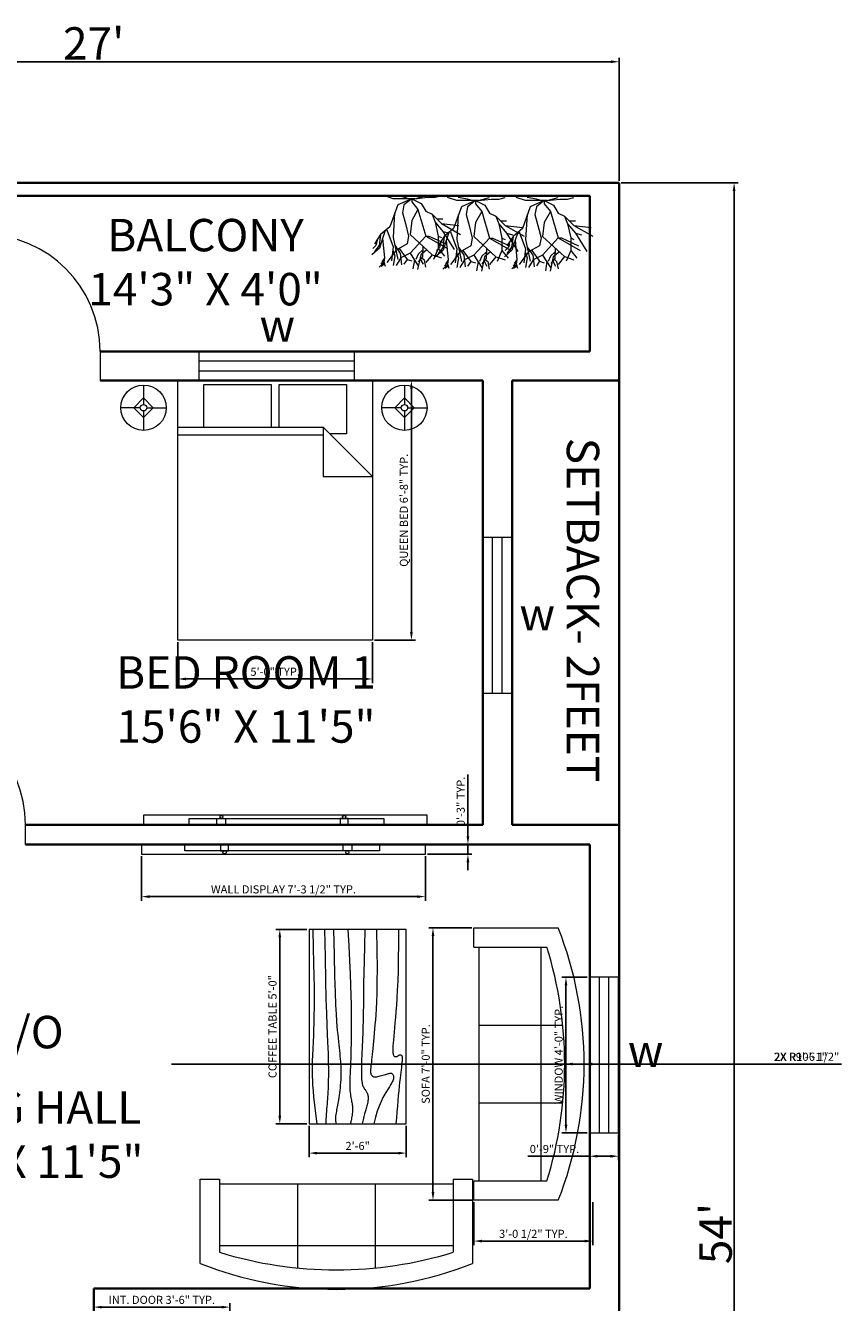
# Model space of a CAD drawing. Units: inches. Extents: x 2729 to 3178, y 5006 to 5809.
# Tile 4 of 4: x 2889 to 3141, y 5415 to 5809. Entities that reach past the tile are written whole.
import ezdxf

# ---------------------------------------------------------------- set-up
doc = ezdxf.new("R2010")
doc.units = ezdxf.units.IN
doc.layers.get('Defpoints').update_dxf_attribs({"color": 72})
for name, color, linetype, lineweight in [('A-ANNO-DIMS', 2, 'Continuous', 18), ('A-ANNO-TEXT', 7, 'Continuous', 18), ('A-AREA-IDEN', 7, 'Continuous', 25), ('A-DOOR', 4, 'Continuous', 18), ('A-EQPM', 8, 'Continuous', 18), ('A-FURN', 8, 'Continuous', 18), ('A-GLAZ', 4, 'Continuous', 18), ('A-WALL', 7, 'Continuous', 35), ('L-PLNT', 72, 'Continuous', 13)]:
    doc.layers.add(name, color=color, linetype=linetype, lineweight=lineweight)
doc.styles.get("Standard").update_dxf_attribs({"font": 'arial.ttf'})
doc.dimstyles.new('ISO-25', dxfattribs={"dimtxt": 2.5, "dimasz": 2.5, "dimexe": 1.25, "dimexo": 0.625, "dimtad": 1, "dimdec": 0, "dimlunit": 3, "dimtxsty": 'Standard', "dimcen": 2.5, "dimadec": 0, "dimazin": 0, "dimtfac": 1, "dimtdec": 0, "dimtmove": 0, "dimatfit": 3, "dimfxl": 1, "dimarcsym": 0})

# ---------------------------------------------------------------- blocks, each defined once
blk = doc.blocks.new('*D1')
at = {"layer": 'A-ANNO-DIMS', "color": 0, "lineweight": -2, "transparency": 16777216}
for p, q in [((2748.18, 5761.26), (2748.18, 5799.21)), ((2750.68, 5797.96), (3069.68, 5797.96)), ((3072.18, 5761.26), (3072.18, 5799.21))]:
    blk.add_line(p, q, dxfattribs=at)
at = {"layer": 'A-ANNO-DIMS', "color": 0, "transparency": 16777216}
for points in [[(2750.68, 5798.38), (2750.68, 5797.54), (2748.18, 5797.96)], [(3069.68, 5798.38), (3069.68, 5797.54), (3072.18, 5797.96)]]:
    blk.add_solid(points, dxfattribs=at)
at = {"layer": 'Defpoints', "color": 0, "transparency": 16777216}
for p in [(3072.18, 5797.96), (2748.18, 5760.64), (3072.18, 5760.64)]:
    blk.add_point(p, dxfattribs=at)
at = {"layer": 'A-ANNO-DIMS', "color": 0, "transparency": 16777216, "insert": (2910.18, 5803.61), "char_height": 2.5, "attachment_point": 5}
blk.add_mtext("{\\H4x;27'}", dxfattribs=at)
blk = doc.blocks.new('*D2')
at = {"layer": 'A-ANNO-DIMS', "color": 0, "lineweight": -2, "transparency": 16777216}
for p, q in [((3072.8, 5760.64), (3108.86, 5760.64)), ((3107.61, 5758.14), (3107.61, 5115.14)), ((3072.8, 5112.64), (3108.86, 5112.64))]:
    blk.add_line(p, q, dxfattribs=at)
at = {"layer": 'A-ANNO-DIMS', "color": 0, "transparency": 16777216}
for points in [[(3107.19, 5758.14), (3108.02, 5758.14), (3107.61, 5760.64)], [(3107.19, 5115.14), (3108.02, 5115.14), (3107.61, 5112.64)]]:
    blk.add_solid(points, dxfattribs=at)
at = {"layer": 'Defpoints', "color": 0, "transparency": 16777216}
for p in [(3072.18, 5760.64), (3072.18, 5112.64), (3107.61, 5112.64)]:
    blk.add_point(p, dxfattribs=at)
at = {"layer": 'A-ANNO-DIMS', "color": 0, "transparency": 16777216, "insert": (3101.9, 5436.64), "char_height": 2.5, "attachment_point": 5, "rotation": 90}
blk.add_mtext("{\\H4x;54'}", dxfattribs=at)
blk = doc.blocks.new('Sofa - Roundback 7 ft.')
for p, q in [((-12.00002, -32.4421), (-12.00003, -6.5971)), ((11.99997, -32.4421), (11.99998, -6.5971)), ((-36.000027, -34), (-36.000027, -11.4696)), ((35.99998, -34), (35.99998, -11.4696)), ((-35.999844, -13.3819), (35.9998, -13.3819)), ((-36.000027, -32.4421), (35.99998, -32.4421))]:
    blk.add_line(p, q)
for points in [[(-36.000027, -34), (-42.000027, -34), (-42.000027, -8)], [(41.99998, -8), (41.99998, -34), (35.99998, -34)]]:
    blk.add_lwpolyline(points)
for centre, radius, start, end in [((0, -114.25), 114.25, 68.43141, 111.5686), ((-0.00001, -127.1968), 121.1968, 72.72033, 107.2797)]:
    blk.add_arc(centre, radius, start, end)
blk = doc.blocks.new('Table - Rectangular Woodgrain 60 x 30 in.')
for p, q in [((0, 0), (0, -30)), ((60, 0), (0, 0)), ((60, -30), (60, 0)), ((0, -30), (60, -30))]:
    blk.add_line(p, q)
for points in [[(0, -2.4), (4.8155, -2.418), (9.0302, -2.4688), (12.709, -2.5477), (15.9167, -2.65), (18.7181, -2.7711), (21.1781, -2.9063), (23.3616, -3.0508), (25.3333, -3.2), (27.1477, -3.3495), (28.8172, -3.4958), (30.3437, -3.636), (31.7291, -3.7667), (32.9756, -3.8849), (34.0849, -3.9875), (35.059, -4.0714), (35.9, -4.1334), (36.6114, -4.1711), (37.2041, -4.1854), (37.6906, -4.1779), (38.0833, -4.15), (38.3948, -4.1034), (38.6375, -4.0396), (38.8239, -3.9602), (38.9666, -3.8667), (39.0764, -3.7608), (39.1573, -3.6448), (39.2116, -3.521), (39.2416, -3.3917), (39.2498, -3.2593), (39.2385, -3.1261), (39.21, -2.9944), (39.1666, -2.8667), (39.111, -2.7447), (39.0468, -2.6281), (38.978, -2.5163), (38.9083, -2.4083), (38.8418, -2.3035), (38.7823, -2.201), (38.7337, -2.1001), (38.7, -2), (38.6844, -1.9003), (38.6875, -1.8021), (38.7094, -1.707), (38.75, -1.6167), (38.8094, -1.5326), (38.8875, -1.4563), (38.9844, -1.3893), (39.1, -1.3333), (39.2351, -1.2896), (39.3937, -1.2583), (39.5804, -1.2396), (39.8, -1.2333), (40.057, -1.2396), (40.3562, -1.2583), (40.7023, -1.2896), (41.1, -1.3333), (41.5547, -1.3895), (42.0755, -1.4573), (42.6721, -1.5361), (43.3542, -1.625), (44.1316, -1.7233), (45.014, -1.8302), (46.0114, -1.9449), (47.1333, -2.0667), (48.3862, -2.1947), (49.7625, -2.3281), (51.2513, -2.4663), (52.8416, -2.6083), (54.5226, -2.7535), (56.2833, -2.9011), (58.1127, -3.0501), (60, -3.2)], [(0, -9.2), (6.5759, -9.0858), (11.9385, -9.0365), (16.2527, -9.0418), (19.6833, -9.0917), (22.3952, -9.1759), (24.5531, -9.2844), (26.322, -9.4069), (27.8666, -9.5333), (29.3241, -9.6553), (30.7203, -9.7719), (32.0532, -9.8837), (33.3208, -9.9917), (34.5213, -10.0965), (35.6526, -10.199), (36.7128, -10.2999), (37.7, -10.4), (38.6129, -10.4996), (39.4531, -10.5969), (40.223, -10.6895), (40.925, -10.775), (41.5613, -10.8512), (42.1344, -10.9156), (42.6465, -10.966), (43.1, -11), (43.4976, -11.0158), (43.8437, -11.0136), (44.143, -10.9942), (44.4, -10.9583), (44.6195, -10.9069), (44.8062, -10.8406), (44.9648, -10.7603), (45.1, -10.6667), (45.2155, -10.5598), (45.3114, -10.4365), (45.3871, -10.2929), (45.4416, -10.125), (45.4743, -9.929), (45.4844, -9.7011), (45.4709, -9.4371), (45.4333, -9.1333), (45.3716, -8.7883), (45.2896, -8.4104), (45.1919, -8.0107), (45.0833, -7.6), (44.9685, -7.1893), (44.8521, -6.7896), (44.7388, -6.4117), (44.6333, -6.0667), (44.54, -5.7628), (44.4614, -5.4979), (44.4001, -5.2675), (44.3583, -5.0667), (44.3384, -4.8909), (44.3427, -4.7354), (44.3736, -4.5956), (44.4333, -4.4667), (44.5236, -4.3453), (44.6427, -4.2333), (44.7884, -4.1339), (44.9583, -4.05), (45.1501, -3.9849), (45.3614, -3.9417), (45.59, -3.9234), (45.8333, -3.9333), (46.0915, -3.9749), (46.3734, -4.0531), (46.6906, -4.1736), (47.0542, -4.3417), (47.4756, -4.5629), (47.9661, -4.8427), (48.5372, -5.1866), (49.2, -5.6), (49.9676, -6.0844), (50.8594, -6.625), (51.8965, -7.2031), (53.1, -7.8), (54.491, -8.3969), (56.0906, -8.975), (57.9199, -9.5156), (60, -10)], [(0, -12.8), (5.1847, -12.9322), (9.6213, -13.0323), (13.3963, -13.1059), (16.5958, -13.1583), (19.3063, -13.1952), (21.614, -13.2219), (23.6054, -13.2439), (25.3666, -13.2667), (26.9728, -13.2947), (28.4531, -13.3281), (29.8256, -13.3663), (31.1083, -13.4083), (32.3191, -13.4535), (33.476, -13.501), (34.597, -13.5501), (35.7, -13.6), (36.7984, -13.6497), (37.8875, -13.6979), (38.9578, -13.743), (40, -13.7833), (41.0047, -13.8174), (41.9625, -13.8438), (42.864, -13.8607), (43.7, -13.8667), (44.4631, -13.8604), (45.1552, -13.8417), (45.7801, -13.8104), (46.3416, -13.7667), (46.8439, -13.7104), (47.2906, -13.6417), (47.6858, -13.5604), (48.0333, -13.4667), (48.3375, -13.3608), (48.6042, -13.2448), (48.8396, -13.121), (49.05, -12.9917), (49.2417, -12.8593), (49.4208, -12.7261), (49.5937, -12.5944), (49.7667, -12.4667), (49.9452, -12.3451), (50.1323, -12.2313), (50.3303, -12.1268), (50.5416, -12.0333), (50.7686, -11.9524), (51.0135, -11.8854), (51.2788, -11.8341), (51.5666, -11.8), (51.8785, -11.7843), (52.2116, -11.7865), (52.562, -11.8059), (52.926, -11.8417), (53.2998, -11.8931), (53.6795, -11.9594), (54.0614, -12.0397), (54.4416, -12.1333), (54.8223, -12.2401), (55.2293, -12.3625), (55.6942, -12.5037), (56.2489, -12.6667), (56.9251, -12.8547), (57.7545, -13.0708), (58.7689, -13.3182), (60, -13.6)], [(0, -18), (5.124, -17.7273), (9.6609, -17.5057), (13.6705, -17.3303), (17.2125, -17.1958), (20.3467, -17.0973), (23.1328, -17.0297), (25.6307, -16.9878), (27.9, -16.9667), (29.9928, -16.9617), (31.9302, -16.9703), (33.7254, -16.9907), (35.3917, -17.0208), (36.9423, -17.0588), (38.3906, -17.1026), (39.7499, -17.1503), (41.0333, -17.2), (42.2519, -17.2496), (43.4073, -17.2969), (44.4986, -17.3395), (45.525, -17.375), (46.4858, -17.4012), (47.3802, -17.4156), (48.2074, -17.416), (48.9667, -17.4), (49.6583, -17.3662), (50.2872, -17.3167), (50.8595, -17.2547), (51.3812, -17.1833), (51.8584, -17.1057), (52.2971, -17.025), (52.7034, -16.9443), (53.0833, -16.8667), (53.443, -16.7951), (53.789, -16.7313), (54.128, -16.6768), (54.4666, -16.6334), (54.8115, -16.6024), (55.1693, -16.5854), (55.5465, -16.5841), (55.95, -16.6), (56.3828, -16.6337), (56.8346, -16.6823), (57.2915, -16.7418), (57.7396, -16.8084), (58.165, -16.878), (58.5539, -16.9469), (58.8924, -17.0111), (59.1666, -17.0667), (59.3679, -17.1107), (59.5078, -17.1438), (59.6032, -17.1675), (59.6708, -17.1833), (59.7275, -17.193), (59.7901, -17.1979), (59.8753, -17.1998), (60, -17.2)], [(0, -22.4), (8.0098, -22.2501), (14.4094, -22.1011), (19.4168, -21.9535), (23.25, -21.8083), (26.1269, -21.6663), (28.2656, -21.5281), (29.884, -21.3947), (31.2, -21.2667), (32.3967, -21.1448), (33.5172, -21.0292), (34.5697, -20.9198), (35.5625, -20.8167), (36.5037, -20.7198), (37.4015, -20.6292), (38.2642, -20.5448), (39.1, -20.4667), (39.9164, -20.3951), (40.7187, -20.3313), (41.5117, -20.2768), (42.3, -20.2333), (43.0883, -20.2024), (43.8812, -20.1854), (44.6836, -20.1841), (45.5, -20.2), (46.3328, -20.234), (47.1747, -20.2844), (48.0163, -20.3488), (48.8479, -20.425), (49.66, -20.5106), (50.4429, -20.6031), (51.1872, -20.7004), (51.8833, -20.8), (52.5246, -20.8999), (53.1166, -20.9995), (53.6681, -21.0983), (54.1875, -21.1958), (54.6834, -21.2919), (55.1646, -21.3859), (55.6394, -21.4777), (56.1167, -21.5667), (56.6028, -21.6515), (57.0961, -21.7266), (57.5929, -21.7852), (58.0896, -21.8208), (58.5823, -21.8268), (59.0674, -21.7964), (59.5412, -21.723), (60, -21.6)], [(0, -25.2), (8.6355, -25.0504), (15.7026, -24.9031), (21.4049, -24.7606), (25.9458, -24.625), (29.529, -24.4988), (32.3578, -24.3844), (34.6359, -24.284), (36.5667, -24.2), (38.3213, -24.1341), (39.9417, -24.0854), (41.437, -24.0523), (42.8167, -24.0333), (44.0901, -24.0268), (45.2667, -24.0313), (46.3557, -24.0451), (47.3667, -24.0667), (48.309, -24.0947), (49.1928, -24.1287), (50.0284, -24.168), (50.826, -24.2125), (51.5959, -24.2617), (52.3483, -24.3151), (53.0935, -24.3725), (53.8417, -24.4334), (54.6009, -24.497), (55.3699, -24.561), (56.1454, -24.6226), (56.9239, -24.6792), (57.7021, -24.7279), (58.4764, -24.7662), (59.2435, -24.7911), (60, -24.8)], [(0, -28.8), (5.6867, -28.6681), (10.45, -28.5698), (14.407, -28.5012), (17.675, -28.4584), (20.3711, -28.4374), (22.6125, -28.4344), (24.5164, -28.4455), (26.2, -28.4667), (27.762, -28.4947), (29.2276, -28.5281), (30.6033, -28.5663), (31.8958, -28.6084), (33.1118, -28.6535), (34.2578, -28.7011), (35.3405, -28.7501), (36.3666, -28.8), (37.3443, -28.8497), (38.288, -28.8974), (39.2137, -28.9412), (40.1375, -28.9792), (41.0753, -29.0093), (42.0432, -29.0297), (43.0572, -29.0384), (44.1333, -29.0333), (45.2936, -29.0114), (46.5843, -28.9641), (48.0579, -28.8816), (49.7666, -28.7542), (51.7629, -28.5721), (54.0989, -28.3255), (56.8272, -28.0048), (60, -27.6)]]:
    blk.add_lwpolyline(points)
blk = doc.blocks.new('Bed - Queen')
for p, q in [((0, -80.00003), (0, 0)), ((0, 0), (59.99999, 0)), ((59.99999, 0), (59.99999, -80.00003)), ((7.99999, -1.2), (28.79998, -1.2)), ((7.99999, -14.4), (7.99999, -1.2)), ((28.79998, -1.2), (28.79998, -14.4)), ((31.19999, -1.2), (51.99999, -1.2)), ((31.19999, -14.4), (31.19999, -1.2)), ((51.99999, -1.2), (51.99999, -16.4)), ((0, -14.4), (44.8, -14.4)), ((59.99999, -29.6), (44.8, -14.4)), ((44.8, -14.4), (44.8, -29.6)), ((44.8, -16.8), (0, -16.8)), ((51.99999, -16.4), (46.79936, -16.4)), ((44.8, -29.6), (59.99999, -29.6)), ((59.99999, -80.00003), (0, -80.00003))]:
    blk.add_line(p, q)
blk = doc.blocks.new('Lamp - Table')
for p, q in [((0, 7), (0, 1)), ((-1, 0), (-7, 0)), ((0, 3), (-3, 0)), ((-3, 0), (0, -3)), ((3, 0), (0, 3)), ((0, -3), (3, 0)), ((1, 0), (7, 0)), ((0, -1), (0, -7))]:
    blk.add_line(p, q)
for radius in [7, 1]:
    blk.add_circle((0, 0), radius)
blk = doc.blocks.new('*U13')
for p, q in [((-377.952, 463.296), (-329.184, 524.256)), ((-316.7634, 502.285), (-327.6092, 559.9176)), ((-296.5958, 484.4034), (-316.7634, 502.285)), ((-286.512, 498.3226), (-307.4416, 538.0736)), ((-302.7934, 478.4344), (-270.256, 518.1854)), ((-290.3982, 464.5406), (-265.6078, 577.8246)), ((-268.7066, 458.5716), (-250.0884, 500.3038)), ((-207.264, 451.104), (-268.224, 548.64)), ((-240.792, 502.285), (-228.3968, 573.8368)), ((-182.88, 499.872), (-219.456, 512.064)), ((-182.88, 499.872), (-158.496, 536.448)), ((-129.1844, 450.6214), (-140.0302, 542.036)), ((-134.112, 487.68), (-97.536, 548.64)), ((-97.536, 426.72), (-24.384, 524.256)), ((-85.7758, 472.4908), (-73.3552, 548.005)), ((-73.152, 402.336), (-60.96, 512.064)), ((-12.9032, 555.9552), (-2.0574, 522.1732)), ((-5.1562, 486.3846), (2.5908, 542.036)), ((-3.6068, 492.3536), (14.986, 518.1854)), ((-0.508, 508.254), (22.7584, 536.067)), ((1.0414, 526.1356), (35.1536, 559.9176)), ((2.5908, 542.036), (21.209, 555.9552)), ((-463.296, 280.416), (-552.577, 423.037)), ((-329.184, 316.992), (-499.872, 414.528)), ((-426.72, 414.528), (-475.488, 475.488)), ((-377.952, 463.296), (-451.104, 487.68)), ((-426.72, 414.528), (-390.144, 499.872)), ((-426.72, 316.992), (-426.72, 414.528)), ((-207.264, 304.8), (-377.952, 463.296)), ((-338.455, 424.7896), (-290.3982, 464.5406)), ((-329.184, 316.992), (-207.264, 451.104)), ((-305.8922, 396.9512), (-302.7934, 478.4344)), ((-304.3428, 426.7708), (-268.7066, 458.5716)), ((-207.264, 451.104), (-134.112, 487.68)), ((-121.92, 414.528), (-182.88, 499.872)), ((-182.88, 377.952), (-97.536, 426.72)), ((-85.7758, 389.001), (-129.1844, 452.6026)), ((-73.152, 329.184), (-109.728, 499.872)), ((-70.2564, 426.7708), (-85.7758, 472.4908)), ((-24.384, 268.224), (-73.152, 402.336)), ((8.7884, 335.3562), (-5.1562, 486.3846)), ((8.7884, 335.3562), (33.6042, 412.8516)), ((33.6042, 412.8516), (92.5068, 464.5406)), ((36.576, 390.144), (73.152, 438.912)), ((60.96, 390.144), (85.344, 414.528)), ((-451.104, 219.456), (-601.0402, 303.8094)), ((-353.568, 316.992), (-487.68, 377.952)), ((-426.72, 316.992), (-451.104, 329.184)), ((-402.336, 207.264), (-426.72, 316.992)), ((-329.184, 316.992), (-353.568, 316.992)), ((-268.224, 109.728), (-329.184, 316.992)), ((-219.456, 195.072), (-207.264, 304.8)), ((-195.072, 316.992), (-182.88, 377.952)), ((-170.688, 219.456), (-195.072, 316.992)), ((-85.344, 134.112), (-73.152, 329.184)), ((-48.768, 243.84), (24.384, 304.8)), ((-12.192, 274.32), (8.7884, 335.3562)), ((24.384, 304.8), (36.576, 390.144)), ((24.384, 304.8), (73.152, 377.952)), ((48.768, 341.376), (60.96, 390.144)), ((-451.104, 219.456), (-587.4512, 234.2388)), ((-463.296, 280.416), (-512.064, 292.608)), ((-402.336, 207.264), (-463.296, 280.416)), ((-377.952, 146.304), (-451.104, 219.456)), ((-377.952, 146.304), (-402.336, 207.264)), ((-146.304, 134.112), (-170.688, 219.456)), ((-109.728, 73.152), (-48.768, 243.84)), ((-414.528, 182.88), (-463.296, 182.88)), ((-329.184, 121.92), (-377.952, 146.304)), ((-292.608, 60.96), (-329.184, 121.92)), ((-268.224, 109.728), (-219.456, 195.072)), ((-219.456, 48.768), (-268.224, 109.728)), ((-158.496, 73.152), (-146.304, 134.112)), ((-402.336, 12.192), (-451.104, 0)), ((-341.376, 12.192), (-402.336, 12.192)), ((-243.84, 24.384), (-341.376, 12.192)), ((-243.84, 24.384), (-329.184, 0)), ((-219.456, 24.384), (-292.608, 60.96)), ((-243.84, 24.384), (-195.072, 24.384)), ((-219.456, 24.384), (-109.728, 73.152)), ((-219.456, 24.384), (-158.496, 73.152)), ((-219.456, 24.384), (-219.456, 48.768)), ((-219.456, 24.384), (-73.152, 24.384)), ((-195.072, 24.384), (-158.496, 12.192)), ((-158.496, 12.192), (-85.344, 0)), ((-73.152, 24.384), (0, 0))]:
    blk.add_line(p, q)
blk = doc.blocks.new('WIN-48IN')
for p, q in [((48, 9), (0, 9)), ((0, 9), (0, 0)), ((48, 0), (48, 9)), ((48, 6), (0, 6)), ((0, 3), (48, 3)), ((0, 0), (48, 0))]:
    blk.add_line(p, q)
blk = doc.blocks.new('DISPLAY-WALL-60IN')
for p, q in [((0, 3), (0, 0)), ((13.37, 1), (13.37, 3)), ((13.37, 3), (73.37, 3)), ((73.37, 1), (13.37, 1)), ((24.34, 3), (24.34, 1)), ((24.34, 1), (26.79, 1)), ((26.79, 1), (26.79, 3)), ((62.14, 1), (62.14, 3)), ((64.8, 1), (62.14, 1)), ((64.8, 3), (64.8, 1)), ((73.37, 3), (73.37, 1)), ((87.48, 0), (87.48, 3)), ((0, 0), (87.48, 0))]:
    blk.add_line(p, q)
for centre, radius in [((25.58, 0.52), 0.492), ((63.4, 0.52), 0.473)]:
    blk.add_circle(centre, radius)
blk = doc.blocks.new('DOOR-36IN-JAMB6')
for p, q in [((0, 6), (0, 42)), ((1, 6), (1, 42)), ((0, 6), (0, 0)), ((1, 6), (1, 0)), ((36, 0), (36, 6))]:
    blk.add_line(p, q)
blk.add_arc((0, 6), 36, 0, 90)
blk = doc.blocks.new('*D27')
at = {"layer": 'A-ANNO-DIMS', "color": 0, "lineweight": -2, "transparency": 16777216}
for p, q in [((3062.36, 5515.67), (3054.53, 5515.67)), ((3055.78, 5470.17), (3055.78, 5513.17)), ((3062.36, 5467.67), (3054.53, 5467.67))]:
    blk.add_line(p, q, dxfattribs=at)
at = {"layer": 'A-ANNO-DIMS', "color": 0, "transparency": 16777216}
for points in [[(3055.37, 5513.17), (3056.2, 5513.17), (3055.78, 5515.67)], [(3055.37, 5470.17), (3056.2, 5470.17), (3055.78, 5467.67)]]:
    blk.add_solid(points, dxfattribs=at)
at = {"layer": 'Defpoints', "color": 0, "transparency": 16777216}
for p in [(3055.78, 5515.67), (3062.98, 5515.67), (3062.98, 5467.67)]:
    blk.add_point(p, dxfattribs=at)
at = {"layer": 'A-ANNO-DIMS', "color": 0, "transparency": 16777216, "insert": (3053.86, 5491.67), "char_height": 2.5, "attachment_point": 5, "rotation": 90}
blk.add_mtext('WINDOW 4\'-0" TYP.', dxfattribs=at)
blk = doc.blocks.new('*D28')
at = {"layer": 'A-ANNO-DIMS', "color": 0, "lineweight": -2, "transparency": 16777216}
for p, q in [((3062.98, 5467.04), (3062.98, 5459.22)), ((3071.98, 5467.04), (3071.98, 5459.22)), ((3062.98, 5460.47), (3043.99, 5460.47)), ((3069.48, 5460.47), (3065.48, 5460.47))]:
    blk.add_line(p, q, dxfattribs=at)
at = {"layer": 'A-ANNO-DIMS', "color": 0, "transparency": 16777216}
for points in [[(3065.48, 5460.89), (3065.48, 5460.05), (3062.98, 5460.47)], [(3069.48, 5460.89), (3069.48, 5460.05), (3071.98, 5460.47)]]:
    blk.add_solid(points, dxfattribs=at)
at = {"layer": 'Defpoints', "color": 0, "transparency": 16777216}
for p in [(3062.98, 5467.67), (3071.98, 5467.67), (3062.98, 5460.47)]:
    blk.add_point(p, dxfattribs=at)
at = {"layer": 'A-ANNO-DIMS', "color": 0, "transparency": 16777216, "insert": (3052.24, 5462.37), "char_height": 2.5, "attachment_point": 5}
blk.add_mtext('0\'-9" TYP.', dxfattribs=at)
blk = doc.blocks.new('*D31')
at = {"layer": 'A-ANNO-DIMS', "color": 0, "lineweight": -2, "transparency": 16777216}
for p, q in [((2996.75, 5699.64), (3009.38, 5699.64)), ((3008.13, 5622.14), (3008.13, 5697.14)), ((2996.75, 5619.64), (3009.38, 5619.64))]:
    blk.add_line(p, q, dxfattribs=at)
at = {"layer": 'A-ANNO-DIMS', "color": 0, "transparency": 16777216}
for points in [[(3007.71, 5697.14), (3008.55, 5697.14), (3008.13, 5699.64)], [(3007.71, 5622.14), (3008.55, 5622.14), (3008.13, 5619.64)]]:
    blk.add_solid(points, dxfattribs=at)
at = {"layer": 'Defpoints', "color": 0, "transparency": 16777216}
for p in [(2996.13, 5699.64), (3008.13, 5699.64), (2996.13, 5619.64)]:
    blk.add_point(p, dxfattribs=at)
at = {"layer": 'A-ANNO-DIMS', "color": 0, "transparency": 16777216, "insert": (3006.13, 5659.64), "char_height": 2.5, "attachment_point": 5, "rotation": 90}
blk.add_mtext('QUEEN BED 6\'-8" TYP.', dxfattribs=at)
blk = doc.blocks.new('*D32')
at = {"layer": 'A-ANNO-DIMS', "color": 0, "lineweight": -2, "transparency": 16777216}
for p, q in [((2936.13, 5619.01), (2936.13, 5606.39)), ((2996.13, 5619.01), (2996.13, 5606.39)), ((2938.63, 5607.64), (2993.63, 5607.64))]:
    blk.add_line(p, q, dxfattribs=at)
at = {"layer": 'A-ANNO-DIMS', "color": 0, "transparency": 16777216}
for points in [[(2938.63, 5608.05), (2938.63, 5607.22), (2936.13, 5607.64)], [(2993.63, 5608.05), (2993.63, 5607.22), (2996.13, 5607.64)]]:
    blk.add_solid(points, dxfattribs=at)
at = {"layer": 'Defpoints', "color": 0, "transparency": 16777216}
for p in [(2936.13, 5619.64), (2996.13, 5619.64), (2996.13, 5607.64)]:
    blk.add_point(p, dxfattribs=at)
at = {"layer": 'A-ANNO-DIMS', "color": 0, "transparency": 16777216, "insert": (2966.13, 5609.54), "char_height": 2.5, "attachment_point": 5}
blk.add_mtext('5\'-0" TYP.', dxfattribs=at)
blk = doc.blocks.new('*D35')
at = {"layer": 'A-ANNO-DIMS', "color": 0, "lineweight": -2, "transparency": 16777216}
for p, q in [((2910.18, 5408.26), (2910.18, 5415.19)), ((2952.18, 5408.26), (2952.18, 5415.19)), ((2912.68, 5413.94), (2949.68, 5413.94))]:
    blk.add_line(p, q, dxfattribs=at)
at = {"layer": 'A-ANNO-DIMS', "color": 0, "transparency": 16777216}
for points in [[(2912.68, 5414.35), (2912.68, 5413.52), (2910.18, 5413.94)], [(2949.68, 5414.35), (2949.68, 5413.52), (2952.18, 5413.94)]]:
    blk.add_solid(points, dxfattribs=at)
at = {"layer": 'Defpoints', "color": 0, "transparency": 16777216}
for p in [(2952.18, 5413.94), (2910.18, 5407.64), (2952.18, 5407.64)]:
    blk.add_point(p, dxfattribs=at)
at = {"layer": 'A-ANNO-DIMS', "color": 0, "transparency": 16777216, "insert": (2931.18, 5415.86), "char_height": 2.5, "attachment_point": 5}
blk.add_mtext('INT. DOOR 3\'-6" TYP.', dxfattribs=at)
blk = doc.blocks.new('*D37')
at = {"layer": 'A-ANNO-DIMS', "color": 0, "lineweight": -2, "transparency": 16777216}
for p, q in [((3026.76, 5530.9), (3013.53, 5530.9)), ((3014.78, 5528.4), (3014.78, 5449.4)), ((3026.76, 5446.9), (3013.53, 5446.9))]:
    blk.add_line(p, q, dxfattribs=at)
at = {"layer": 'A-ANNO-DIMS', "color": 0, "transparency": 16777216}
for points in [[(3014.37, 5528.4), (3015.2, 5528.4), (3014.78, 5530.9)], [(3014.37, 5449.4), (3015.2, 5449.4), (3014.78, 5446.9)]]:
    blk.add_solid(points, dxfattribs=at)
at = {"layer": 'Defpoints', "color": 0, "transparency": 16777216}
for p in [(3027.38, 5530.9), (3014.78, 5446.9), (3027.38, 5446.9)]:
    blk.add_point(p, dxfattribs=at)
at = {"layer": 'A-ANNO-DIMS', "color": 0, "transparency": 16777216, "insert": (3012.87, 5488.9), "char_height": 2.5, "attachment_point": 5, "rotation": 90}
blk.add_mtext('SOFA 7\'-0" TYP.', dxfattribs=at)
blk = doc.blocks.new('*D38')
at = {"layer": 'A-ANNO-DIMS', "color": 0, "lineweight": -2, "transparency": 16777216}
for p, q in [((3027.38, 5446.27), (3027.38, 5433.05)), ((3064.05, 5446.27), (3064.05, 5433.05)), ((3029.88, 5434.3), (3061.55, 5434.3))]:
    blk.add_line(p, q, dxfattribs=at)
at = {"layer": 'A-ANNO-DIMS', "color": 0, "transparency": 16777216}
for points in [[(3029.88, 5434.72), (3029.88, 5433.88), (3027.38, 5434.3)], [(3061.55, 5434.72), (3061.55, 5433.88), (3064.05, 5434.3)]]:
    blk.add_solid(points, dxfattribs=at)
at = {"layer": 'Defpoints', "color": 0, "transparency": 16777216}
for p in [(3027.38, 5446.9), (3064.05, 5446.9), (3064.05, 5434.3)]:
    blk.add_point(p, dxfattribs=at)
at = {"layer": 'A-ANNO-DIMS', "color": 0, "transparency": 16777216, "insert": (3045.72, 5436.22), "char_height": 2.5, "attachment_point": 5}
blk.add_mtext('3\'-0 1/2" TYP.', dxfattribs=at)
blk = doc.blocks.new('*D43')
at = {"layer": 'A-ANNO-DIMS', "color": 0, "lineweight": -2, "transparency": 16777216}
for p, q in [((2924.96, 5553.01), (2924.96, 5539.27)), ((3012.43, 5553.01), (3012.43, 5539.27)), ((2927.46, 5540.52), (3009.93, 5540.52))]:
    blk.add_line(p, q, dxfattribs=at)
at = {"layer": 'A-ANNO-DIMS', "color": 0, "transparency": 16777216}
for points in [[(2927.46, 5540.93), (2927.46, 5540.1), (2924.96, 5540.52)], [(3009.93, 5540.93), (3009.93, 5540.1), (3012.43, 5540.52)]]:
    blk.add_solid(points, dxfattribs=at)
at = {"layer": 'Defpoints', "color": 0, "transparency": 16777216}
for p in [(2924.96, 5553.64), (3012.43, 5553.64), (3012.43, 5540.52)]:
    blk.add_point(p, dxfattribs=at)
at = {"layer": 'A-ANNO-DIMS', "color": 0, "transparency": 16777216, "insert": (2968.69, 5542.43), "char_height": 2.5, "attachment_point": 5}
blk.add_mtext('WALL DISPLAY 7\'-3 1/2" TYP.', dxfattribs=at)
blk = doc.blocks.new('*D44')
at = {"layer": 'A-ANNO-DIMS', "color": 0, "lineweight": -2, "transparency": 16777216}
for p, q in [((3025.55, 5559.14), (3025.55, 5578.13)), ((3013.06, 5556.64), (3026.8, 5556.64)), ((3025.55, 5553.64), (3025.55, 5556.64)), ((3013.06, 5553.64), (3026.8, 5553.64)), ((3025.55, 5551.14), (3025.55, 5548.64))]:
    blk.add_line(p, q, dxfattribs=at)
at = {"layer": 'A-ANNO-DIMS', "color": 0, "transparency": 16777216}
for points in [[(3025.14, 5559.14), (3025.97, 5559.14), (3025.55, 5556.64)], [(3025.14, 5551.14), (3025.97, 5551.14), (3025.55, 5553.64)]]:
    blk.add_solid(points, dxfattribs=at)
at = {"layer": 'Defpoints', "color": 0, "transparency": 16777216}
for p in [(3012.43, 5556.64), (3025.55, 5556.64), (3012.43, 5553.64)]:
    blk.add_point(p, dxfattribs=at)
at = {"layer": 'A-ANNO-DIMS', "color": 0, "transparency": 16777216, "insert": (3023.65, 5569.88), "char_height": 2.5, "attachment_point": 5, "rotation": 90}
blk.add_mtext('0\'-3" TYP.', dxfattribs=at)
blk = doc.blocks.new('*D49')
at = {"layer": 'A-ANNO-DIMS', "color": 0, "lineweight": -2, "transparency": 16777216}
for p, q in [((2975.93, 5530.43), (2966.31, 5530.43)), ((2967.56, 5527.93), (2967.56, 5472.93)), ((2975.93, 5470.43), (2966.31, 5470.43))]:
    blk.add_line(p, q, dxfattribs=at)
at = {"layer": 'A-ANNO-DIMS', "color": 0, "transparency": 16777216}
for points in [[(2967.14, 5527.93), (2967.97, 5527.93), (2967.56, 5530.43)], [(2967.14, 5472.93), (2967.97, 5472.93), (2967.56, 5470.43)]]:
    blk.add_solid(points, dxfattribs=at)
at = {"layer": 'Defpoints', "color": 0, "transparency": 16777216}
for p in [(2976.56, 5530.43), (2967.56, 5470.43), (2976.56, 5470.43)]:
    blk.add_point(p, dxfattribs=at)
at = {"layer": 'A-ANNO-DIMS', "color": 0, "transparency": 16777216, "insert": (2965.64, 5500.43), "char_height": 2.5, "attachment_point": 5, "rotation": 90}
blk.add_mtext('COFFEE TABLE 5\'-0"', dxfattribs=at)
blk = doc.blocks.new('*D50')
at = {"layer": 'A-ANNO-DIMS', "color": 0, "lineweight": -2, "transparency": 16777216}
for p, q in [((2976.56, 5469.8), (2976.56, 5460.18)), ((3006.56, 5469.8), (3006.56, 5460.18)), ((2979.06, 5461.43), (3004.06, 5461.43))]:
    blk.add_line(p, q, dxfattribs=at)
at = {"layer": 'A-ANNO-DIMS', "color": 0, "transparency": 16777216}
for points in [[(2979.06, 5461.84), (2979.06, 5461.01), (2976.56, 5461.43)], [(3004.06, 5461.84), (3004.06, 5461.01), (3006.56, 5461.43)]]:
    blk.add_solid(points, dxfattribs=at)
at = {"layer": 'Defpoints', "color": 0, "transparency": 16777216}
for p in [(2976.56, 5470.43), (3006.56, 5470.43), (3006.56, 5461.43)]:
    blk.add_point(p, dxfattribs=at)
at = {"layer": 'A-ANNO-DIMS', "color": 0, "transparency": 16777216, "insert": (2991.56, 5463.33), "char_height": 2.5, "attachment_point": 5}
blk.add_mtext('2\'-6"', dxfattribs=at)
blk = doc.blocks.new('*D56')
at = {"layer": 'A-ANNO-DIMS', "color": 0, "lineweight": -2, "transparency": 16777216}
for p, q in [((2934.19, 5488.9), (3055.38, 5488.9)), ((3136.93, 5488.9), (3057.88, 5488.9))]:
    blk.add_line(p, q, dxfattribs=at)
at = {"layer": 'A-ANNO-DIMS', "color": 0, "transparency": 16777216}
blk.add_solid([(3057.88, 5489.32), (3057.88, 5488.48), (3055.38, 5488.9)], dxfattribs=at)
at = {"layer": 'Defpoints', "color": 0, "transparency": 16777216}
for p in [(2934.19, 5488.9), (3055.38, 5488.9)]:
    blk.add_point(p, dxfattribs=at)
at = {"layer": 'A-ANNO-DIMS', "color": 0, "transparency": 16777216, "insert": (3128.1, 5490.8), "char_height": 2.5, "attachment_point": 5, "rotation": 359.9998}
blk.add_mtext('2X R10\'-1"', dxfattribs=at)
blk = doc.blocks.new('*D57')
at = {"layer": 'A-ANNO-DIMS', "color": 0, "lineweight": -2, "transparency": 16777216}
for p, q in [((2947.13, 5488.9), (3061.38, 5488.9)), ((3140.7, 5488.9), (3063.88, 5488.9))]:
    blk.add_line(p, q, dxfattribs=at)
at = {"layer": 'A-ANNO-DIMS', "color": 0, "transparency": 16777216}
blk.add_solid([(3063.88, 5489.32), (3063.88, 5488.48), (3061.38, 5488.9)], dxfattribs=at)
at = {"layer": 'Defpoints', "color": 0, "transparency": 16777216}
for p in [(2947.13, 5488.9), (3061.38, 5488.9)]:
    blk.add_point(p, dxfattribs=at)
at = {"layer": 'A-ANNO-DIMS', "color": 0, "transparency": 16777216, "insert": (3129.93, 5490.82), "char_height": 2.5, "attachment_point": 5, "rotation": 359.9998}
blk.add_mtext('2X R9\'-6 1/2"', dxfattribs=at)

msp = doc.modelspace()

# ---------------------------------------------------------------- linework, layer by layer
at = {"layer": 'A-DOOR'}
msp.add_line((2912.18, 5708.64), (2912.18, 5699.64), dxfattribs=at)
msp.add_arc((2876.18, 5708.64), 36, 0, 90, dxfattribs=at)
at = {"layer": 'A-WALL'}
for p, q in [((2748.18, 5760.64), (3072.18, 5760.64)), ((3072.18, 5760.64), (3072.18, 5112.64)), ((3072.18, 5760.64), (3072.18, 5112.64)), ((2757.18, 5756.64), (3063.18, 5756.64)), ((3063.18, 5756.64), (3063.18, 5708.64)), ((2912.18, 5708.64), (3063.18, 5708.64)), ((2912.18, 5699.64), (3030.18, 5699.64)), ((3030.18, 5699.64), (3030.18, 5562.64)), ((3039.18, 5699.64), (3039.18, 5562.64)), ((3039.18, 5699.64), (3072.18, 5699.64)), ((2889.18, 5562.64), (3030.18, 5562.64)), ((3039.18, 5562.64), (3072.18, 5562.64)), ((2889.18, 5556.64), (3063.18, 5556.64)), ((3063.18, 5556.64), (3063.18, 5419.64)), ((3063.18, 5556.64), (3063.18, 5419.64)), ((2910.18, 5419.64), (3063.18, 5419.64)), ((2910.18, 5419.64), (2910.18, 5407.64))]:
    msp.add_line(p, q, dxfattribs=at)

# ---------------------------------------------------------------- block references
at = {"layer": 'A-DOOR'}
msp.add_blockref('DOOR-36IN-JAMB6', (2853.18, 5556.64), dxfattribs=at)
at = {"layer": 'A-EQPM', "rotation": 180}
msp.add_blockref('DISPLAY-WALL-60IN', (3012.97, 5565.63), dxfattribs=at)
at = {"layer": 'A-EQPM'}
msp.add_blockref('DISPLAY-WALL-60IN', (2924.96, 5553.64), dxfattribs=at)
at = {"layer": 'A-FURN'}
for name, p in [('Lamp - Table', (2925.56, 5691.28)), ('Bed - Queen', (2936.13, 5699.64)), ('Lamp - Table', (3005.97, 5691.28))]:
    msp.add_blockref(name, p, dxfattribs=at)
for name, p, rotation in [('Table - Rectangular Woodgrain 60 x 30 in.', (3006.56, 5530.43), 270), ('Sofa - Roundback 7 ft.', (3061.38, 5488.9), 270), ('Sofa - Roundback 7 ft.', (2985, 5419.41), 180)]:
    msp.add_blockref(name, p, dxfattribs=dict(at, rotation=rotation))
at = {"layer": 'A-GLAZ'}
msp.add_blockref('WIN-48IN', (2942.55, 5699.64), dxfattribs=at)
for p, rotation in [((3039.06, 5603.21), 90.00000000000003), ((3071.98, 5467.67), 89.99999999999856)]:
    msp.add_blockref('WIN-48IN', p, dxfattribs=dict(at, rotation=rotation))
at = {"layer": 'L-PLNT', "xscale": 0.0393700787401575, "yscale": 0.0393700787401575, "zscale": 0.0393700787401575, "rotation": 180}
for p in [(2999.6, 5756.69), (3019.23, 5756.09), (3040.43, 5756.11)]:
    msp.add_blockref('*U13', p, dxfattribs=at)

# ---------------------------------------------------------------- texts
at = {"layer": 'A-ANNO-TEXT', "char_height": 10, "attachment_point": 1}
for s, width, insert in [('w', 11.1436, (2961.32, 5721.65)), ('w', 11.1436, (3041.45, 5632.62)), ('\\pxqc;A/O', 28.8912, (2874.59, 5503.75)), ('w', 11.1436, (3074.86, 5498.02))]:
    msp.add_mtext_dynamic_manual_height_columns(s, width=width, gutter_width=12.5, heights=[0], dxfattribs=dict(at, insert=insert))
at = {"layer": 'A-ANNO-TEXT', "insert": (3066.02, 5694.09), "char_height": 10, "attachment_point": 1, "rotation": 270}
msp.add_mtext_dynamic_manual_height_columns('\\pxqc;SETBACK- 2FEET', width=130.3517, gutter_width=12.5, heights=[0], dxfattribs=at)
at = {"layer": 'A-AREA-IDEN', "char_height": 10, "attachment_point": 1}
for s, width, insert in [('\\pxqc;BALCONY \\P14\'3" X 4\'0"', 73.4706, (2907.93, 5749.5)), ('\\pxqc;BED ROOM 1\\P15\'6" X 11\'5"', 111.1664, (2901.54, 5614.65)), ('\\pxqc;LIVING HALL\\P18\'9" X 11\'5"', 114.8323, (2828.17, 5480.46))]:
    msp.add_mtext_dynamic_manual_height_columns(s, width=width, gutter_width=12.5, heights=[0], dxfattribs=dict(at, insert=insert))

# ---------------------------------------------------------------- dimensions: what is measured, and where the dimension line sits
at = {"layer": 'A-ANNO-DIMS'}
for base, p1, p2, text, override, picture, middle in [((3072.18, 5797.96), (2748.18, 5760.64), (3072.18, 5760.64), "{\\H4x;27'}", {"dimclrd": 0, "dimclre": 0, "dimclrt": 0}, '*D1', (2910.18, 5803.61)), ((2996.13, 5607.64), (2936.13, 5619.64), (2996.13, 5619.64), '<> TYP.', {"dimdec": 1, "dimlfac": 1, "dimrnd": 0, "dimzin": 1, "dimdsep": 46, "dimlunit": 4, "dimfrac": 2}, '*D32', (2966.13, 5609.54)), ((3012.43, 5540.52), (2924.96, 5553.64), (3012.43, 5553.64), 'WALL DISPLAY <> TYP.', {"dimdec": 1, "dimlfac": 1, "dimrnd": 0, "dimzin": 1, "dimdsep": 46, "dimlunit": 4, "dimfrac": 2}, '*D43', (2968.69, 5542.43)), ((3064.05, 5434.3), (3027.38, 5446.9), (3064.05, 5446.9), '<> TYP.', {"dimdec": 1, "dimlfac": 1, "dimrnd": 0, "dimzin": 1, "dimdsep": 46, "dimlunit": 4, "dimfrac": 2}, '*D38', (3045.72, 5436.22)), ((2952.18, 5413.94), (2910.18, 5407.64), (2952.18, 5407.64), 'INT. DOOR <> TYP.', {"dimdec": 1, "dimlfac": 1, "dimrnd": 0, "dimzin": 1, "dimdsep": 46, "dimlunit": 4, "dimfrac": 2}, '*D35', (2931.18, 5415.86))]:
    dim = msp.add_linear_dim(base=base, p1=p1, p2=p2, text=text, dimstyle='ISO-25', override=override, dxfattribs=at)
    dim.commit()
    dim.dimension.update_dxf_attribs({"geometry": picture, "text_midpoint": middle})
for base, p1, p2, angle, text, override, picture, middle in [((3107.61, 5112.64), (3072.18, 5760.64), (3072.18, 5112.64), 90, "{\\H4x;54'}", {"dimclrd": 0, "dimclre": 0, "dimclrt": 0}, '*D2', (3101.9, 5436.64)), ((3008.13, 5699.64), (2996.13, 5619.64), (2996.13, 5699.64), 90, 'QUEEN BED <> TYP.', {"dimdec": 1, "dimlfac": 1, "dimrnd": 0, "dimzin": 1, "dimdsep": 46, "dimlunit": 4, "dimfrac": 2}, '*D31', (3006.13, 5659.64)), ((3025.55, 5556.64), (3012.43, 5553.64), (3012.43, 5556.64), 90, '<> TYP.', {"dimdec": 1, "dimlfac": 1, "dimrnd": 0, "dimzin": 1, "dimdsep": 46, "dimlunit": 4, "dimfrac": 2}, '*D44', (3023.65, 5569.88)), ((2967.56, 5470.43), (2976.56, 5530.43), (2976.56, 5470.43), 270, 'COFFEE TABLE <>', {"dimdec": 1, "dimlfac": 1, "dimrnd": 0, "dimzin": 1, "dimdsep": 46, "dimlunit": 4, "dimfrac": 2}, '*D49', (2965.64, 5500.43)), ((3014.78, 5446.9), (3027.38, 5530.9), (3027.38, 5446.9), 270, 'SOFA <> TYP.', {"dimdec": 1, "dimlfac": 1, "dimrnd": 0, "dimzin": 1, "dimdsep": 46, "dimlunit": 4, "dimfrac": 2}, '*D37', (3012.87, 5488.9)), ((3055.78, 5515.67), (3062.98, 5467.67), (3062.98, 5515.67), 90, 'WINDOW <> TYP.', {"dimdec": 1, "dimlfac": 1, "dimrnd": 0, "dimzin": 1, "dimdsep": 46, "dimlunit": 4, "dimfrac": 2}, '*D27', (3053.86, 5491.67)), ((3062.98, 5460.47), (3071.98, 5467.67), (3062.98, 5467.67), 180, '<> TYP.', {"dimdec": 1, "dimlfac": 1, "dimrnd": 0, "dimzin": 1, "dimdsep": 46, "dimlunit": 4, "dimfrac": 2}, '*D28', (3052.24, 5462.37))]:
    dim = msp.add_linear_dim(base=base, p1=p1, p2=p2, angle=angle, text=text, dimstyle='ISO-25', override=override, dxfattribs=at)
    dim.commit()
    dim.dimension.update_dxf_attribs({"geometry": picture, "text_midpoint": middle})
for center, mpoint, picture, middle in [((2934.19, 5488.9), (3055.38, 5488.9), '*D56', (3128.1, 5488.9)), ((2947.134784, 5488.899342), (3061.384784, 5488.899), '*D57', (3129.934784, 5488.8987948))]:
    dim = msp.add_radius_dim(center=center, mpoint=mpoint, text='2X <>', dimstyle='ISO-25', override={"dimdec": 1, "dimlfac": 1, "dimrnd": 0, "dimzin": 1, "dimdsep": 46, "dimlunit": 4, "dimfrac": 2}, dxfattribs=at)
    dim.commit()
    dim.dimension.update_dxf_attribs({"geometry": picture, "text_midpoint": middle, "dimtype": 164})
dim = msp.add_linear_dim(base=(3006.56, 5461.43), p1=(2976.56, 5470.43), p2=(3006.56, 5470.43), dimstyle='ISO-25', override={"dimdec": 1, "dimlfac": 1, "dimrnd": 0, "dimzin": 1, "dimdsep": 46, "dimlunit": 4, "dimfrac": 2}, dxfattribs=at)
dim.commit()
dim.dimension.update_dxf_attribs({"geometry": '*D50', "text_midpoint": (2991.56, 5463.33)})

doc.saveas('drawing.dxf')
